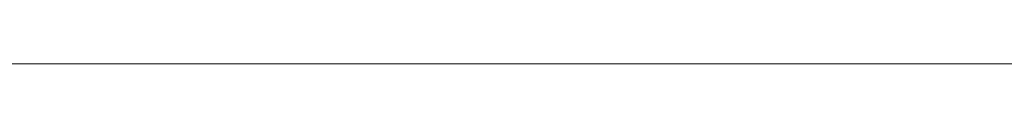
# Model space of a CAD drawing. Units: inches. Extents: x 459864 to 460310, y 324185 to 324787.
# Tile 87 of 112: x 460247.12218 to 460247.14006, y 324283.48322 to 324283.48324. Entities that reach past the tile are written whole.
import ezdxf

# ---------------------------------------------------------------- set-up
doc = ezdxf.new("R2010")
doc.units = ezdxf.units.IN
for name, color, linetype, lineweight in [('A-ANNO-DIMS', 2, 'Continuous', 18), ('L-HRDS', 9, 'Continuous', 18), ('L-SITE-PATT', 252, 'Continuous', 13)]:
    doc.layers.add(name, color=color, linetype=linetype, lineweight=lineweight)
doc.styles.get("Standard").update_dxf_attribs({"font": 'arial.ttf'})
doc.dimstyles.new('ISO-25', dxfattribs={"dimtxt": 6, "dimasz": 2.5, "dimexe": 1.25, "dimexo": 0.625, "dimtad": 1, "dimdec": 1, "dimlunit": 3, "dimtxsty": 'Standard', "dimcen": 2.5, "dimadec": 0, "dimazin": 0, "dimtfac": 1, "dimtdec": 1, "dimtmove": 0, "dimatfit": 3, "dimfxl": 1, "dimarcsym": 0})

# ---------------------------------------------------------------- blocks, each defined once
blk = doc.blocks.new('*D21')
at = {"layer": 'A-ANNO-DIMS', "color": 0, "lineweight": -2, "transparency": 16777216}
for p, q in [((460247.739927, 324715.483233), (460309.580369, 324715.483233)), ((460308.330369, 324712.983233), (460308.330369, 324285.983233)), ((460247.739927, 324283.483233), (460309.580369, 324283.483233))]:
    blk.add_line(p, q, dxfattribs=at)
at = {"layer": 'A-ANNO-DIMS', "color": 0, "transparency": 16777216}
for points in [[(460307.913702, 324712.983233), (460308.747035, 324712.983233), (460308.330369, 324715.483233)], [(460307.913702, 324285.983233), (460308.747035, 324285.983233), (460308.330369, 324283.483233)]]:
    blk.add_solid(points, dxfattribs=at)
at = {"layer": 'Defpoints', "color": 0, "transparency": 16777216}
for p in [(460247.114927, 324715.483233), (460247.114927, 324283.483233), (460308.330369, 324283.483233)]:
    blk.add_point(p, dxfattribs=at)
at = {"layer": 'A-ANNO-DIMS', "color": 0, "transparency": 16777216, "insert": (460304.639884, 324499.483233), "char_height": 6, "attachment_point": 5, "rotation": 90}
blk.add_mtext("36'", dxfattribs=at)

msp = doc.modelspace()

# ---------------------------------------------------------------- hatches: boundary and pattern name
at = {"layer": 'L-SITE-PATT'}
h = msp.add_hatch(dxfattribs=at)
h.set_pattern_fill('DOTS', color=256)
h.paths.add_polyline_path([(460269.803614, 324283.483233), (460247.114927, 324283.483233), (460121.929275, 324283.483233), (460121.929275, 324252.47302), (460117.429275, 324252.47302), (460110.123563, 324252.47302), (460110.123563, 324243.286537), (460080.829543, 324243.286537), (460080.829543, 324252.47302), (460061.114927, 324252.47302), (460061.114927, 324251.882422), (460077.9089, 324251.882422), (460077.9089, 324199.483233), (460080.829543, 324199.483233), (460080.829543, 324207.553216), (460110.123563, 324207.553216), (460110.123563, 324199.483233), (460110.813349, 324199.483233), (460262.114927, 324199.483233), (460269.803614, 324199.483233)], flags=17)
edge = h.paths.add_edge_path(flags=0)
edge.add_ellipse((460222.590295, 324263.813229), major_axis=(-8.485281, 8.485281), ratio=1, start_angle=405, end_angle=495, ccw=False)
edge.add_line((460214.820868, 324254.65989), (460214.831619, 324254.66592))
edge.add_ellipse((460222.590295, 324263.813229), major_axis=(-8.485281, 8.485281), ratio=1, start_angle=405, end_angle=495, ccw=False)
edge.add_line((460210.75891, 324261.780551), (460210.767583, 324261.786823))
edge.add_ellipse((460222.590295, 324263.813229), major_axis=(-8.485281, 8.485281), ratio=1, start_angle=405, end_angle=495, ccw=False)
edge.add_ellipse((460222.590295, 324263.813229), major_axis=(-8.485281, 8.485281), ratio=1, start_angle=392.754016, end_angle=405, ccw=False)
edge.add_ellipse((460222.590295, 324263.813229), major_axis=(-8.485281, 8.485281), ratio=1, start_angle=380.9347178, end_angle=392.754016, ccw=False)
edge.add_line((460211.337059, 324267.985029), (460211.340404, 324267.985029))
edge.add_ellipse((460222.590295, 324263.813229), major_axis=(-8.485281, 8.485281), ratio=1, start_angle=380.9347178, end_angle=392.754016, ccw=False)
edge.add_ellipse((460222.590295, 324263.813229), major_axis=(-8.485281, 8.485281), ratio=1, start_angle=347.9015209, end_angle=380.9347178, ccw=False)
edge.add_ellipse((460222.590295, 324263.813229), major_axis=(-8.485281, 8.485281), ratio=1, start_angle=327.0619241, end_angle=347.9015209, ccw=False)
edge.add_ellipse((460222.590295, 324263.813229), major_axis=(-8.485281, 8.485281), ratio=1, start_angle=278.3246418, end_angle=327.0619241, ccw=False)
edge.add_line((460225.158278, 324275.535991), (460225.157699, 324275.534637))
edge.add_ellipse((460222.590295, 324263.813229), major_axis=(-8.485281, 8.485281), ratio=1, start_angle=278.3246418, end_angle=327.0619241, ccw=False)
edge.add_ellipse((460222.590295, 324263.813229), major_axis=(-8.485281, 8.485281), ratio=1, start_angle=260.6435685, end_angle=278.3246418, ccw=False)
edge.add_ellipse((460222.590295, 324263.813229), major_axis=(-8.485281, 8.485281), ratio=1, start_angle=225, end_angle=260.6435685, ccw=False)
edge.add_line((460234.508791, 324265.242796), (460234.501456, 324265.239441))
edge.add_ellipse((460222.590295, 324263.813229), major_axis=(-8.485281, 8.485281), ratio=1, start_angle=225, end_angle=260.6435685, ccw=False)
edge.add_ellipse((460222.590295, 324263.813229), major_axis=(-8.485281, 8.485281), ratio=1, start_angle=495, end_angle=585, ccw=False)
edge.add_line((460234.436668, 324261.861215), (460234.423783, 324261.857822))
edge.add_ellipse((460222.590295, 324263.813229), major_axis=(-8.485281, 8.485281), ratio=1, start_angle=495, end_angle=585, ccw=False)
edge.add_line((460227.95013, 324253.067192), (460227.946414, 324253.083139))
edge.add_ellipse((460222.590295, 324263.813229), major_axis=(-8.485281, 8.485281), ratio=1, start_angle=495, end_angle=585, ccw=False)
edge.add_line((460226.222975, 324252.369267), (460226.21103, 324252.379551))
edge.add_ellipse((460222.590295, 324263.813229), major_axis=(-8.485281, 8.485281), ratio=1, start_angle=495, end_angle=585, ccw=False)
h.paths.add_polyline_path([(460219.651452, 324254.346654), (460218.461311, 324253.544985), (460218.275437, 324254.78932), (460219.642395, 324256.541765), (460219.62463, 324260.847564), (460216.110089, 324257.333022), (460214.349967, 324256.978066), (460215.416366, 324259.355678), (460212.523935, 324258.495823), (460213.137313, 324259.929797), (460218.507211, 324263.813229), (460222.590295, 324263.813229), (460222.590295, 324267.806698), (460218.175536, 324272.21231), (460219.025968, 324274.63898), (460222.590295, 324272.811129), (460222.590295, 324275.42332), (460223.057099, 324274.824931), (460222.67523, 324273.492211), (460225.911677, 324267.134611), (460219.62463, 324260.847564)], flags=0)
edge = h.paths.add_edge_path(flags=0)
edge.add_ellipse((460194.575758, 324264.046494), major_axis=(-8.485281, 8.485281), ratio=1, start_angle=495, end_angle=585, ccw=False)
edge.add_line((460199.935593, 324253.300458), (460199.931877, 324253.316405))
edge.add_ellipse((460194.575758, 324264.046494), major_axis=(-8.485281, 8.485281), ratio=1, start_angle=495, end_angle=585, ccw=False)
edge.add_line((460198.208438, 324252.602533), (460198.196493, 324252.612817))
edge.add_ellipse((460194.575758, 324264.046494), major_axis=(-8.485281, 8.485281), ratio=1, start_angle=495, end_angle=585, ccw=False)
edge.add_ellipse((460194.575758, 324264.046494), major_axis=(-8.485281, 8.485281), ratio=1, start_angle=405, end_angle=495, ccw=False)
edge.add_line((460186.806331, 324254.893156), (460186.817082, 324254.899186))
edge.add_ellipse((460194.575758, 324264.046494), major_axis=(-8.485281, 8.485281), ratio=1, start_angle=405, end_angle=495, ccw=False)
edge.add_line((460182.744373, 324262.013817), (460182.753046, 324262.020089))
edge.add_ellipse((460194.575758, 324264.046494), major_axis=(-8.485281, 8.485281), ratio=1, start_angle=405, end_angle=495, ccw=False)
edge.add_ellipse((460194.575758, 324264.046494), major_axis=(-8.485281, 8.485281), ratio=1, start_angle=392.754016, end_angle=405, ccw=False)
edge.add_ellipse((460194.575758, 324264.046494), major_axis=(-8.485281, 8.485281), ratio=1, start_angle=380.9347178, end_angle=392.754016, ccw=False)
edge.add_line((460183.322522, 324268.218294), (460183.325867, 324268.218294))
edge.add_ellipse((460194.575758, 324264.046494), major_axis=(-8.485281, 8.485281), ratio=1, start_angle=380.9347178, end_angle=392.754016, ccw=False)
edge.add_ellipse((460194.575758, 324264.046494), major_axis=(-8.485281, 8.485281), ratio=1, start_angle=347.9015209, end_angle=380.9347178, ccw=False)
edge.add_ellipse((460194.575758, 324264.046494), major_axis=(-8.485281, 8.485281), ratio=1, start_angle=327.0619241, end_angle=347.9015209, ccw=False)
edge.add_ellipse((460194.575758, 324264.046494), major_axis=(-8.485281, 8.485281), ratio=1, start_angle=278.3246418, end_angle=327.0619241, ccw=False)
edge.add_line((460197.143741, 324275.769257), (460197.143162, 324275.767903))
edge.add_ellipse((460194.575758, 324264.046494), major_axis=(-8.485281, 8.485281), ratio=1, start_angle=278.3246418, end_angle=327.0619241, ccw=False)
edge.add_ellipse((460194.575758, 324264.046494), major_axis=(-8.485281, 8.485281), ratio=1, start_angle=260.6435685, end_angle=278.3246418, ccw=False)
edge.add_ellipse((460194.575758, 324264.046494), major_axis=(-8.485281, 8.485281), ratio=1, start_angle=225, end_angle=260.6435685, ccw=False)
edge.add_line((460206.494254, 324265.476062), (460206.486919, 324265.472707))
edge.add_ellipse((460194.575758, 324264.046494), major_axis=(-8.485281, 8.485281), ratio=1, start_angle=225, end_angle=260.6435685, ccw=False)
edge.add_ellipse((460194.575758, 324264.046494), major_axis=(-8.485281, 8.485281), ratio=1, start_angle=495, end_angle=585, ccw=False)
edge.add_line((460206.422132, 324262.094481), (460206.409246, 324262.091088))
h.paths.add_polyline_path([(460191.610093, 324261.08083), (460191.636915, 324254.57992), (460190.446774, 324253.778251), (460190.2609, 324255.022585), (460191.627858, 324256.775031), (460191.610093, 324261.08083), (460188.095552, 324257.566288), (460186.33543, 324257.211332), (460187.40183, 324259.588944), (460184.509398, 324258.729088), (460185.122776, 324260.163063), (460190.492675, 324264.046494), (460194.575758, 324264.046494), (460194.575758, 324268.039963), (460190.160999, 324272.445576), (460191.011431, 324274.872246), (460194.575758, 324273.044395), (460194.575758, 324275.656585), (460195.042562, 324275.058197), (460194.660693, 324273.725477), (460197.897141, 324267.367877)], flags=0)
edge = h.paths.add_edge_path(flags=0)
edge.add_ellipse((460252.911961, 324263.577616), major_axis=(-8.485281, 8.485281), ratio=1, start_angle=405, end_angle=495, ccw=False)
edge.add_line((460241.080576, 324261.544938), (460241.089249, 324261.55121))
edge.add_ellipse((460252.911961, 324263.577616), major_axis=(-8.485281, 8.485281), ratio=1, start_angle=405, end_angle=495, ccw=False)
edge.add_ellipse((460252.911961, 324263.577616), major_axis=(-8.485281, 8.485281), ratio=1, start_angle=392.754016, end_angle=405, ccw=False)
edge.add_ellipse((460252.911961, 324263.577616), major_axis=(-8.485281, 8.485281), ratio=1, start_angle=380.9347178, end_angle=392.754016, ccw=False)
edge.add_line((460241.658725, 324267.749416), (460241.66207, 324267.749416))
edge.add_ellipse((460252.911961, 324263.577616), major_axis=(-8.485281, 8.485281), ratio=1, start_angle=380.9347178, end_angle=392.754016, ccw=False)
edge.add_ellipse((460252.911961, 324263.577616), major_axis=(-8.485281, 8.485281), ratio=1, start_angle=347.9015209, end_angle=380.9347178, ccw=False)
edge.add_ellipse((460252.911961, 324263.577616), major_axis=(-8.485281, 8.485281), ratio=1, start_angle=327.0619241, end_angle=347.9015209, ccw=False)
edge.add_ellipse((460252.911961, 324263.577616), major_axis=(-8.485281, 8.485281), ratio=1, start_angle=278.3246418, end_angle=327.0619241, ccw=False)
edge.add_line((460255.479944, 324275.300378), (460255.479365, 324275.299024))
edge.add_ellipse((460252.911961, 324263.577616), major_axis=(-8.485281, 8.485281), ratio=1, start_angle=278.3246418, end_angle=327.0619241, ccw=False)
edge.add_ellipse((460252.911961, 324263.577616), major_axis=(-8.485281, 8.485281), ratio=1, start_angle=260.6435685, end_angle=278.3246418, ccw=False)
edge.add_ellipse((460252.911961, 324263.577616), major_axis=(-8.485281, 8.485281), ratio=1, start_angle=225, end_angle=260.6435685, ccw=False)
edge.add_line((460264.830457, 324265.007183), (460264.823122, 324265.003828))
edge.add_ellipse((460252.911961, 324263.577616), major_axis=(-8.485281, 8.485281), ratio=1, start_angle=225, end_angle=260.6435685, ccw=False)
edge.add_ellipse((460252.911961, 324263.577616), major_axis=(-8.485281, 8.485281), ratio=1, start_angle=495, end_angle=585, ccw=False)
edge.add_line((460264.758335, 324261.625602), (460264.745449, 324261.622209))
edge.add_ellipse((460252.911961, 324263.577616), major_axis=(-8.485281, 8.485281), ratio=1, start_angle=495, end_angle=585, ccw=False)
edge.add_line((460258.271796, 324252.831579), (460258.268081, 324252.847526))
edge.add_ellipse((460252.911961, 324263.577616), major_axis=(-8.485281, 8.485281), ratio=1, start_angle=495, end_angle=585, ccw=False)
edge.add_line((460256.544641, 324252.133654), (460256.532696, 324252.143938))
edge.add_ellipse((460252.911961, 324263.577616), major_axis=(-8.485281, 8.485281), ratio=1, start_angle=495, end_angle=585, ccw=False)
edge.add_ellipse((460252.911961, 324263.577616), major_axis=(-8.485281, 8.485281), ratio=1, start_angle=405, end_angle=495, ccw=False)
edge.add_line((460245.142534, 324254.424277), (460245.153285, 324254.430307))
h.paths.add_polyline_path([(460244.671633, 324256.742453), (460245.738033, 324259.120065), (460242.845601, 324258.26021), (460243.458979, 324259.694184), (460248.828878, 324263.577616), (460252.911961, 324263.577616), (460252.911961, 324267.571085), (460248.497202, 324271.976697), (460249.347634, 324274.403367), (460252.911961, 324272.575516), (460252.911961, 324275.187707), (460253.378765, 324274.589318), (460252.996897, 324273.256598), (460256.233344, 324266.898998), (460249.946296, 324260.611951), (460249.973118, 324254.111041), (460248.782977, 324253.309372), (460248.597103, 324254.553707), (460249.964061, 324256.306152), (460249.946296, 324260.611951), (460246.431755, 324257.097409)], flags=0)
edge = h.paths.add_edge_path(flags=0)
edge.add_ellipse((460167.43869, 324262.832792), major_axis=(-8.485281, 8.485281), ratio=1, start_angle=495, end_angle=585, ccw=False)
edge.add_line((460172.798524, 324252.086755), (460172.794809, 324252.102702))
edge.add_ellipse((460167.43869, 324262.832792), major_axis=(-8.485281, 8.485281), ratio=1, start_angle=495, end_angle=585, ccw=False)
edge.add_line((460171.07137, 324251.38883), (460171.059425, 324251.399114))
edge.add_ellipse((460167.43869, 324262.832792), major_axis=(-8.485281, 8.485281), ratio=1, start_angle=495, end_angle=585, ccw=False)
edge.add_ellipse((460167.43869, 324262.832792), major_axis=(-8.485281, 8.485281), ratio=1, start_angle=405, end_angle=495, ccw=False)
edge.add_line((460159.669262, 324253.679453), (460159.680013, 324253.685483))
edge.add_ellipse((460167.43869, 324262.832792), major_axis=(-8.485281, 8.485281), ratio=1, start_angle=405, end_angle=495, ccw=False)
edge.add_line((460155.607304, 324260.800114), (460155.615977, 324260.806386))
edge.add_ellipse((460167.43869, 324262.832792), major_axis=(-8.485281, 8.485281), ratio=1, start_angle=405, end_angle=495, ccw=False)
edge.add_ellipse((460167.43869, 324262.832792), major_axis=(-8.485281, 8.485281), ratio=1, start_angle=392.754016, end_angle=405, ccw=False)
edge.add_ellipse((460167.43869, 324262.832792), major_axis=(-8.485281, 8.485281), ratio=1, start_angle=380.9347178, end_angle=392.754016, ccw=False)
edge.add_line((460156.185453, 324267.004592), (460156.188798, 324267.004592))
edge.add_ellipse((460167.43869, 324262.832792), major_axis=(-8.485281, 8.485281), ratio=1, start_angle=380.9347178, end_angle=392.754016, ccw=False)
edge.add_ellipse((460167.43869, 324262.832792), major_axis=(-8.485281, 8.485281), ratio=1, start_angle=347.9015209, end_angle=380.9347178, ccw=False)
edge.add_ellipse((460167.43869, 324262.832792), major_axis=(-8.485281, 8.485281), ratio=1, start_angle=327.0619241, end_angle=347.9015209, ccw=False)
edge.add_ellipse((460167.43869, 324262.832792), major_axis=(-8.485281, 8.485281), ratio=1, start_angle=278.3246418, end_angle=327.0619241, ccw=False)
edge.add_line((460170.006672, 324274.555554), (460170.006093, 324274.5542))
edge.add_ellipse((460167.43869, 324262.832792), major_axis=(-8.485281, 8.485281), ratio=1, start_angle=278.3246418, end_angle=327.0619241, ccw=False)
edge.add_ellipse((460167.43869, 324262.832792), major_axis=(-8.485281, 8.485281), ratio=1, start_angle=260.6435685, end_angle=278.3246418, ccw=False)
edge.add_ellipse((460167.43869, 324262.832792), major_axis=(-8.485281, 8.485281), ratio=1, start_angle=225, end_angle=260.6435685, ccw=False)
edge.add_line((460179.357186, 324264.262359), (460179.349851, 324264.259004))
edge.add_ellipse((460167.43869, 324262.832792), major_axis=(-8.485281, 8.485281), ratio=1, start_angle=225, end_angle=260.6435685, ccw=False)
edge.add_ellipse((460167.43869, 324262.832792), major_axis=(-8.485281, 8.485281), ratio=1, start_angle=495, end_angle=585, ccw=False)
edge.add_line((460179.285063, 324260.880778), (460179.272177, 324260.877385))
h.paths.add_polyline_path([(460164.473025, 324259.867127), (460164.499846, 324253.366217), (460163.309706, 324252.564548), (460163.123831, 324253.808883), (460164.49079, 324255.561328), (460164.473025, 324259.867127), (460160.958483, 324256.352585), (460159.198362, 324255.997629), (460160.264761, 324258.375241), (460157.372329, 324257.515386), (460157.985707, 324258.94936), (460163.355606, 324262.832792), (460167.43869, 324262.832792), (460167.43869, 324266.826261), (460163.02393, 324271.231873), (460163.874362, 324273.658543), (460167.43869, 324271.830692), (460167.43869, 324274.442883), (460167.905493, 324273.844494), (460167.523625, 324272.511774), (460170.760072, 324266.154174)], flags=0)
edge = h.paths.add_edge_path(flags=0)
edge.add_ellipse((460140.758089, 324262.369585), major_axis=(-8.485281, 8.485281), ratio=1, start_angle=495, end_angle=585, ccw=False)
edge.add_line((460146.117923, 324251.623548), (460146.114208, 324251.639495))
edge.add_ellipse((460140.758089, 324262.369585), major_axis=(-8.485281, 8.485281), ratio=1, start_angle=495, end_angle=585, ccw=False)
edge.add_line((460144.390769, 324250.925623), (460144.378824, 324250.935907))
edge.add_ellipse((460140.758089, 324262.369585), major_axis=(-8.485281, 8.485281), ratio=1, start_angle=495, end_angle=585, ccw=False)
edge.add_ellipse((460140.758089, 324262.369585), major_axis=(-8.485281, 8.485281), ratio=1, start_angle=405, end_angle=495, ccw=False)
edge.add_line((460132.988661, 324253.216246), (460132.999412, 324253.222276))
edge.add_ellipse((460140.758089, 324262.369585), major_axis=(-8.485281, 8.485281), ratio=1, start_angle=405, end_angle=495, ccw=False)
edge.add_line((460128.926703, 324260.336907), (460128.935376, 324260.343179))
edge.add_ellipse((460140.758089, 324262.369585), major_axis=(-8.485281, 8.485281), ratio=1, start_angle=405, end_angle=495, ccw=False)
edge.add_ellipse((460140.758089, 324262.369585), major_axis=(-8.485281, 8.485281), ratio=1, start_angle=392.754016, end_angle=405, ccw=False)
edge.add_ellipse((460140.758089, 324262.369585), major_axis=(-8.485281, 8.485281), ratio=1, start_angle=380.9347178, end_angle=392.754016, ccw=False)
edge.add_line((460129.504852, 324266.541385), (460129.508197, 324266.541385))
edge.add_ellipse((460140.758089, 324262.369585), major_axis=(-8.485281, 8.485281), ratio=1, start_angle=380.9347178, end_angle=392.754016, ccw=False)
edge.add_ellipse((460140.758089, 324262.369585), major_axis=(-8.485281, 8.485281), ratio=1, start_angle=347.9015209, end_angle=380.9347178, ccw=False)
edge.add_ellipse((460140.758089, 324262.369585), major_axis=(-8.485281, 8.485281), ratio=1, start_angle=327.0619241, end_angle=347.9015209, ccw=False)
edge.add_ellipse((460140.758089, 324262.369585), major_axis=(-8.485281, 8.485281), ratio=1, start_angle=278.3246418, end_angle=327.0619241, ccw=False)
edge.add_line((460143.326071, 324274.092347), (460143.325492, 324274.090993))
edge.add_ellipse((460140.758089, 324262.369585), major_axis=(-8.485281, 8.485281), ratio=1, start_angle=278.3246418, end_angle=327.0619241, ccw=False)
edge.add_ellipse((460140.758089, 324262.369585), major_axis=(-8.485281, 8.485281), ratio=1, start_angle=260.6435685, end_angle=278.3246418, ccw=False)
edge.add_ellipse((460140.758089, 324262.369585), major_axis=(-8.485281, 8.485281), ratio=1, start_angle=225, end_angle=260.6435685, ccw=False)
edge.add_line((460152.676585, 324263.799152), (460152.66925, 324263.795797))
edge.add_ellipse((460140.758089, 324262.369585), major_axis=(-8.485281, 8.485281), ratio=1, start_angle=225, end_angle=260.6435685, ccw=False)
edge.add_ellipse((460140.758089, 324262.369585), major_axis=(-8.485281, 8.485281), ratio=1, start_angle=495, end_angle=585, ccw=False)
edge.add_line((460152.604462, 324260.417571), (460152.591576, 324260.414178))
h.paths.add_polyline_path([(460137.792424, 324259.40392), (460137.819245, 324252.90301), (460136.629105, 324252.101341), (460136.44323, 324253.345676), (460137.810189, 324255.098121), (460137.792424, 324259.40392), (460134.277882, 324255.889378), (460132.517761, 324255.534422), (460133.58416, 324257.912034), (460130.691728, 324257.052179), (460131.305106, 324258.486153), (460136.675005, 324262.369585), (460140.758089, 324262.369585), (460140.758089, 324266.363054), (460136.343329, 324270.768666), (460137.193761, 324273.195336), (460140.758089, 324271.367485), (460140.758089, 324273.979676), (460141.224892, 324273.381287), (460140.843024, 324272.048567), (460144.079471, 324265.690967)], flags=0)
h.paths.add_polyline_path([(460110.123563, 324227.413868), (460080.829543, 324227.413868), (460080.829543, 324235.483851), (460110.123563, 324235.483851)], flags=16)
h.paths.add_polyline_path([(460110.123563, 324220.796634), (460110.123563, 324212.726651), (460080.829543, 324212.726651), (460080.829543, 324220.796634)], flags=16)
h.paths.add_polyline_path([(460269.803614, 324283.483233), (460247.114927, 324283.483233), (460121.929275, 324283.483233), (460121.929275, 324252.47302), (460117.429275, 324252.47302), (460110.123563, 324252.47302), (460110.123563, 324243.286537), (460080.829543, 324243.286537), (460080.829543, 324252.47302), (460061.114927, 324252.47302), (460061.114927, 324251.882422), (460077.9089, 324251.882422), (460077.9089, 324199.483233), (460080.829543, 324199.483233), (460080.829543, 324207.553216), (460110.123563, 324207.553216), (460110.123563, 324199.483233), (460262.114927, 324199.483233), (460269.803614, 324199.483233)], flags=17)
h.paths.add_polyline_path([(460219.651452, 324254.346654), (460218.461311, 324253.544985), (460218.275437, 324254.78932), (460219.642395, 324256.541765), (460219.62463, 324260.847564), (460216.110089, 324257.333022), (460214.349967, 324256.978066), (460215.416366, 324259.355678), (460212.523935, 324258.495823), (460213.137313, 324259.929797), (460218.507211, 324263.813229), (460222.590295, 324263.813229), (460220.180486, 324266.223037), (460215.460959, 324265.307646), (460211.834533, 324266.136551), (460216.246619, 324267.985029), (460218.418495, 324267.985029), (460222.590295, 324263.813229), (460222.590295, 324267.806698), (460218.175536, 324272.21231), (460219.025968, 324274.63898), (460222.590295, 324272.811129), (460222.590295, 324275.42332), (460223.057099, 324274.824931), (460222.67523, 324273.492211), (460225.911677, 324267.134611), (460222.590295, 324263.813229), (460231.382871, 324263.813229), (460228.484718, 324262.487825), (460224.425208, 324261.978316), (460228.679899, 324257.723625), (460228.965835, 324254.791014), (460227.141768, 324256.536632), (460227.542067, 324254.818575), (460227.333342, 324253.614466), (460222.590295, 324259.984626), (460222.590295, 324255.496666), (460221.377409, 324256.540849), (460220.575794, 324261.798728), (460219.62463, 324260.847564)], flags=0)
h.paths.add_polyline_path([(460199.127231, 324256.769898), (460199.52753, 324255.051841), (460199.318805, 324253.847732), (460194.575758, 324260.217892), (460194.575758, 324255.729932), (460193.362872, 324256.774115), (460192.561257, 324262.031993), (460191.610093, 324261.08083), (460191.636915, 324254.57992), (460190.446774, 324253.778251), (460190.2609, 324255.022585), (460191.627858, 324256.775031), (460191.610093, 324261.08083), (460188.095552, 324257.566288), (460186.33543, 324257.211332), (460187.40183, 324259.588944), (460184.509398, 324258.729088), (460185.122776, 324260.163063), (460190.492675, 324264.046494), (460194.575758, 324264.046494), (460192.16595, 324266.456303), (460187.446422, 324265.540912), (460183.819996, 324266.369816), (460188.232082, 324268.218294), (460190.403958, 324268.218294), (460194.575758, 324264.046494), (460194.575758, 324268.039963), (460190.160999, 324272.445576), (460191.011431, 324274.872246), (460194.575758, 324273.044395), (460194.575758, 324275.656585), (460195.042562, 324275.058197), (460194.660693, 324273.725477), (460197.897141, 324267.367877), (460194.575758, 324264.046494), (460203.368334, 324264.046494), (460200.470181, 324262.721091), (460196.410671, 324262.211582), (460200.665362, 324257.956891), (460200.951298, 324255.02428)], flags=0)
h.paths.add_polyline_path([(460244.671633, 324256.742453), (460245.738033, 324259.120065), (460242.845601, 324258.26021), (460243.458979, 324259.694184), (460248.828878, 324263.577616), (460252.911961, 324263.577616), (460250.502153, 324265.987424), (460245.782625, 324265.072033), (460242.156199, 324265.900938), (460246.568285, 324267.749416), (460248.740161, 324267.749416), (460252.911961, 324263.577616), (460252.911961, 324267.571085), (460248.497202, 324271.976697), (460249.347634, 324274.403367), (460252.911961, 324272.575516), (460252.911961, 324275.187707), (460253.378765, 324274.589318), (460252.996897, 324273.256598), (460256.233344, 324266.898998), (460252.911961, 324263.577616), (460261.704537, 324263.577616), (460258.806384, 324262.252212), (460254.746874, 324261.742703), (460259.001565, 324257.488012), (460259.287501, 324254.555401), (460257.463434, 324256.301019), (460257.863733, 324254.582962), (460257.655008, 324253.378853), (460252.911961, 324259.749013), (460252.911961, 324255.261053), (460251.699075, 324256.305236), (460250.89746, 324261.563115), (460249.946296, 324260.611951), (460249.973118, 324254.111041), (460248.782977, 324253.309372), (460248.597103, 324254.553707), (460249.964061, 324256.306152), (460249.946296, 324260.611951), (460246.431755, 324257.097409)], flags=0)
h.paths.add_polyline_path([(460173.528293, 324256.743188), (460173.81423, 324253.810577), (460171.990163, 324255.556195), (460172.390461, 324253.838138), (460172.181736, 324252.634029), (460167.43869, 324259.004189), (460167.43869, 324254.516229), (460166.225803, 324255.560412), (460165.424189, 324260.818291), (460164.473025, 324259.867127), (460164.499846, 324253.366217), (460163.309706, 324252.564548), (460163.123831, 324253.808883), (460164.49079, 324255.561328), (460164.473025, 324259.867127), (460160.958483, 324256.352585), (460159.198362, 324255.997629), (460160.264761, 324258.375241), (460157.372329, 324257.515386), (460157.985707, 324258.94936), (460163.355606, 324262.832792), (460167.43869, 324262.832792), (460165.028881, 324265.2426), (460160.309353, 324264.327209), (460156.682927, 324265.156114), (460161.095013, 324267.004592), (460163.26689, 324267.004592), (460167.43869, 324262.832792), (460167.43869, 324266.826261), (460163.02393, 324271.231873), (460163.874362, 324273.658543), (460167.43869, 324271.830692), (460167.43869, 324274.442883), (460167.905493, 324273.844494), (460167.523625, 324272.511774), (460170.760072, 324266.154174), (460167.43869, 324262.832792), (460176.231266, 324262.832792), (460173.333113, 324261.507388), (460169.273603, 324260.997879)], flags=0)
h.paths.add_polyline_path([(460146.847692, 324256.279981), (460147.133629, 324253.34737), (460145.309562, 324255.092988), (460145.70986, 324253.374931), (460145.501135, 324252.170822), (460140.758089, 324258.540983), (460140.758089, 324254.053022), (460139.545202, 324255.097205), (460138.743588, 324260.355084), (460137.792424, 324259.40392), (460137.819245, 324252.90301), (460136.629105, 324252.101341), (460136.44323, 324253.345676), (460137.810189, 324255.098121), (460137.792424, 324259.40392), (460134.277882, 324255.889378), (460132.517761, 324255.534422), (460133.58416, 324257.912034), (460130.691728, 324257.052179), (460131.305106, 324258.486153), (460136.675005, 324262.369585), (460140.758089, 324262.369585), (460138.34828, 324264.779393), (460133.628752, 324263.864002), (460130.002326, 324264.692907), (460134.414412, 324266.541385), (460136.586289, 324266.541385), (460140.758089, 324262.369585), (460140.758089, 324266.363054), (460136.343329, 324270.768666), (460137.193761, 324273.195336), (460140.758089, 324271.367485), (460140.758089, 324273.979676), (460141.224892, 324273.381287), (460140.843024, 324272.048567), (460144.079471, 324265.690967), (460140.758089, 324262.369585), (460149.550664, 324262.369585), (460146.652512, 324261.044182), (460142.593002, 324260.534672)], flags=0)
edge = h.paths.add_edge_path()
edge.add_line((460269.803614, 324272.549054), (460260.881484, 324272.549054))
edge.add_ellipse((460252.911961, 324263.577616), major_axis=(-8.485281, 8.485281), ratio=1, start_angle=260.6435685, end_angle=273.3846244, ccw=False)
edge.add_line((460262.282614, 324271.092108), (460262.260554, 324271.09106))
edge.add_ellipse((460252.911961, 324263.577616), major_axis=(-8.485281, 8.485281), ratio=1, start_angle=260.6435685, end_angle=273.3846244, ccw=False)
edge.add_ellipse((460252.911961, 324263.577616), major_axis=(-8.485281, 8.485281), ratio=1, start_angle=225, end_angle=260.6435685, ccw=False)
edge.add_line((460263.608568, 324269.063294), (460263.571652, 324269.058283))
edge.add_ellipse((460252.911961, 324263.577616), major_axis=(-8.485281, 8.485281), ratio=1, start_angle=225, end_angle=260.6435685, ccw=False)
edge.add_line((460264.615462, 324266.30554), (460264.585358, 324266.305196))
edge.add_ellipse((460252.911961, 324263.577616), major_axis=(-8.485281, 8.485281), ratio=1, start_angle=225, end_angle=260.6435685, ccw=False)
edge.add_line((460264.830457, 324265.007183), (460264.823122, 324265.003828))
edge.add_ellipse((460252.911961, 324263.577616), major_axis=(-8.485281, 8.485281), ratio=1, start_angle=225, end_angle=260.6435685, ccw=False)
edge.add_ellipse((460252.911961, 324263.577616), major_axis=(-8.485281, 8.485281), ratio=1, start_angle=495, end_angle=585, ccw=False)
edge.add_line((460264.758335, 324261.625602), (460264.745449, 324261.622209))
edge.add_ellipse((460252.911961, 324263.577616), major_axis=(-8.485281, 8.485281), ratio=1, start_angle=495, end_angle=585, ccw=False)
edge.add_line((460263.442202, 324257.739018), (460263.389259, 324257.779239))
edge.add_ellipse((460252.911961, 324263.577616), major_axis=(-8.485281, 8.485281), ratio=1, start_angle=495, end_angle=585, ccw=False)
edge.add_line((460258.128071, 324252.743505), (460258.101878, 324252.778683))
edge.add_ellipse((460252.911961, 324263.577616), major_axis=(-8.485281, 8.485281), ratio=1, start_angle=495, end_angle=585, ccw=False)
edge.add_line((460256.544641, 324252.133654), (460256.532696, 324252.143938))
edge.add_ellipse((460252.911961, 324263.577616), major_axis=(-8.485281, 8.485281), ratio=1, start_angle=495, end_angle=585, ccw=False)
edge.add_ellipse((460252.911961, 324263.577616), major_axis=(-8.485281, 8.485281), ratio=1, start_angle=405, end_angle=495, ccw=False)
edge.add_line((460250.593989, 324251.780412), (460250.604653, 324251.819817))
edge.add_ellipse((460252.911961, 324263.577616), major_axis=(-8.485281, 8.485281), ratio=1, start_angle=405, end_angle=495, ccw=False)
edge.add_line((460245.142534, 324254.424277), (460245.153285, 324254.430307))
edge.add_ellipse((460252.911961, 324263.577616), major_axis=(-8.485281, 8.485281), ratio=1, start_angle=405, end_angle=495, ccw=False)
edge.add_line((460243.524588, 324256.059004), (460243.560343, 324256.091361))
edge.add_ellipse((460252.911961, 324263.577616), major_axis=(-8.485281, 8.485281), ratio=1, start_angle=405, end_angle=495, ccw=False)
edge.add_line((460241.440103, 324259.892726), (460241.522441, 324259.895877))
edge.add_ellipse((460252.911961, 324263.577616), major_axis=(-8.485281, 8.485281), ratio=1, start_angle=405, end_angle=495, ccw=False)
edge.add_line((460241.080576, 324261.544938), (460241.089249, 324261.55121))
edge.add_ellipse((460252.911961, 324263.577616), major_axis=(-8.485281, 8.485281), ratio=1, start_angle=405, end_angle=495, ccw=False)
edge.add_ellipse((460252.911961, 324263.577616), major_axis=(-8.485281, 8.485281), ratio=1, start_angle=392.754016, end_angle=405, ccw=False)
edge.add_line((460241.050299, 324265.437612), (460241.062566, 324265.442751))
edge.add_ellipse((460252.911961, 324263.577616), major_axis=(-8.485281, 8.485281), ratio=1, start_angle=392.754016, end_angle=405, ccw=False)
edge.add_ellipse((460252.911961, 324263.577616), major_axis=(-8.485281, 8.485281), ratio=1, start_angle=380.9347178, end_angle=392.754016, ccw=False)
edge.add_line((460241.451888, 324267.176391), (460241.469044, 324267.170988))
edge.add_ellipse((460252.911961, 324263.577616), major_axis=(-8.485281, 8.485281), ratio=1, start_angle=380.9347178, end_angle=392.754016, ccw=False)
edge.add_line((460241.658725, 324267.749416), (460241.66207, 324267.749416))
edge.add_ellipse((460252.911961, 324263.577616), major_axis=(-8.485281, 8.485281), ratio=1, start_angle=380.9347178, end_angle=392.754016, ccw=False)
edge.add_ellipse((460252.911961, 324263.577616), major_axis=(-8.485281, 8.485281), ratio=1, start_angle=356.6153756, end_angle=380.9347178, ccw=False)
edge.add_line((460244.880293, 324272.487651), (460244.712651, 324272.549054))
edge.add_line((460244.712651, 324272.549054), (460230.817406, 324272.549054))
edge.add_ellipse((460222.590295, 324263.813229), major_axis=(-8.485281, 8.485281), ratio=1, start_angle=260.6435685, end_angle=271.7177746, ccw=False)
edge.add_ellipse((460222.590295, 324263.813229), major_axis=(-8.485281, 8.485281), ratio=1, start_angle=225, end_angle=260.6435685, ccw=False)
edge.add_line((460233.286902, 324269.298907), (460233.249986, 324269.293896))
edge.add_ellipse((460222.590295, 324263.813229), major_axis=(-8.485281, 8.485281), ratio=1, start_angle=225, end_angle=260.6435685, ccw=False)
edge.add_line((460234.293796, 324266.541153), (460234.263692, 324266.540809))
edge.add_ellipse((460222.590295, 324263.813229), major_axis=(-8.485281, 8.485281), ratio=1, start_angle=225, end_angle=260.6435685, ccw=False)
edge.add_line((460234.508791, 324265.242796), (460234.501456, 324265.239441))
edge.add_ellipse((460222.590295, 324263.813229), major_axis=(-8.485281, 8.485281), ratio=1, start_angle=225, end_angle=260.6435685, ccw=False)
edge.add_ellipse((460222.590295, 324263.813229), major_axis=(-8.485281, 8.485281), ratio=1, start_angle=495, end_angle=585, ccw=False)
edge.add_line((460234.436668, 324261.861215), (460234.423783, 324261.857822))
edge.add_ellipse((460222.590295, 324263.813229), major_axis=(-8.485281, 8.485281), ratio=1, start_angle=495, end_angle=585, ccw=False)
edge.add_line((460233.120535, 324257.974631), (460233.067593, 324258.014852))
edge.add_ellipse((460222.590295, 324263.813229), major_axis=(-8.485281, 8.485281), ratio=1, start_angle=495, end_angle=585, ccw=False)
edge.add_line((460227.806405, 324252.979118), (460227.780212, 324253.014296))
edge.add_ellipse((460222.590295, 324263.813229), major_axis=(-8.485281, 8.485281), ratio=1, start_angle=495, end_angle=585, ccw=False)
edge.add_line((460226.222975, 324252.369267), (460226.21103, 324252.379551))
edge.add_ellipse((460222.590295, 324263.813229), major_axis=(-8.485281, 8.485281), ratio=1, start_angle=495, end_angle=585, ccw=False)
edge.add_ellipse((460222.590295, 324263.813229), major_axis=(-8.485281, 8.485281), ratio=1, start_angle=405, end_angle=495, ccw=False)
edge.add_line((460220.272323, 324252.016025), (460220.282987, 324252.05543))
edge.add_ellipse((460222.590295, 324263.813229), major_axis=(-8.485281, 8.485281), ratio=1, start_angle=405, end_angle=495, ccw=False)
edge.add_line((460214.820868, 324254.65989), (460214.831619, 324254.66592))
edge.add_ellipse((460222.590295, 324263.813229), major_axis=(-8.485281, 8.485281), ratio=1, start_angle=405, end_angle=495, ccw=False)
edge.add_line((460213.202922, 324256.294617), (460213.238677, 324256.326974))
edge.add_ellipse((460222.590295, 324263.813229), major_axis=(-8.485281, 8.485281), ratio=1, start_angle=405, end_angle=495, ccw=False)
edge.add_line((460211.118437, 324260.128339), (460211.200774, 324260.13149))
edge.add_ellipse((460222.590295, 324263.813229), major_axis=(-8.485281, 8.485281), ratio=1, start_angle=405, end_angle=495, ccw=False)
edge.add_line((460210.75891, 324261.780551), (460210.767583, 324261.786823))
edge.add_ellipse((460222.590295, 324263.813229), major_axis=(-8.485281, 8.485281), ratio=1, start_angle=405, end_angle=495, ccw=False)
edge.add_ellipse((460222.590295, 324263.813229), major_axis=(-8.485281, 8.485281), ratio=1, start_angle=392.754016, end_angle=405, ccw=False)
edge.add_line((460210.728633, 324265.673225), (460210.7409, 324265.678364))
edge.add_ellipse((460222.590295, 324263.813229), major_axis=(-8.485281, 8.485281), ratio=1, start_angle=392.754016, end_angle=405, ccw=False)
edge.add_ellipse((460222.590295, 324263.813229), major_axis=(-8.485281, 8.485281), ratio=1, start_angle=380.9347178, end_angle=392.754016, ccw=False)
edge.add_line((460211.130222, 324267.412004), (460211.147378, 324267.406601))
edge.add_ellipse((460222.590295, 324263.813229), major_axis=(-8.485281, 8.485281), ratio=1, start_angle=380.9347178, end_angle=392.754016, ccw=False)
edge.add_line((460211.337059, 324267.985029), (460211.340404, 324267.985029))
edge.add_ellipse((460222.590295, 324263.813229), major_axis=(-8.485281, 8.485281), ratio=1, start_angle=380.9347178, end_angle=392.754016, ccw=False)
edge.add_ellipse((460222.590295, 324263.813229), major_axis=(-8.485281, 8.485281), ratio=1, start_angle=358.2822254, end_angle=380.9347178, ccw=False)
edge.add_line((460213.704522, 324271.901826), (460213.709044, 324271.868974))
edge.add_ellipse((460222.590295, 324263.813229), major_axis=(-8.485281, 8.485281), ratio=1, start_angle=358.2822254, end_angle=380.9347178, ccw=False)
edge.add_line((460214.363185, 324272.549054), (460203.078318, 324272.549054))
edge.add_line((460203.078318, 324272.549054), (460203.060342, 324272.531078))
edge.add_ellipse((460194.575758, 324264.046494), major_axis=(-8.485281, 8.485281), ratio=1, start_angle=260.6435685, end_angle=270.11679, ccw=False)
edge.add_line((460203.956591, 324271.56147), (460203.920907, 324271.559776))
edge.add_ellipse((460194.575758, 324264.046494), major_axis=(-8.485281, 8.485281), ratio=1, start_angle=260.6435685, end_angle=270.11679, ccw=False)
edge.add_ellipse((460194.575758, 324264.046494), major_axis=(-8.485281, 8.485281), ratio=1, start_angle=225, end_angle=260.6435685, ccw=False)
edge.add_line((460205.272365, 324269.532172), (460205.235449, 324269.527161))
edge.add_ellipse((460194.575758, 324264.046494), major_axis=(-8.485281, 8.485281), ratio=1, start_angle=225, end_angle=260.6435685, ccw=False)
edge.add_line((460206.279259, 324266.774419), (460206.249155, 324266.774075))
edge.add_ellipse((460194.575758, 324264.046494), major_axis=(-8.485281, 8.485281), ratio=1, start_angle=225, end_angle=260.6435685, ccw=False)
edge.add_line((460206.494254, 324265.476062), (460206.486919, 324265.472707))
edge.add_ellipse((460194.575758, 324264.046494), major_axis=(-8.485281, 8.485281), ratio=1, start_angle=225, end_angle=260.6435685, ccw=False)
edge.add_ellipse((460194.575758, 324264.046494), major_axis=(-8.485281, 8.485281), ratio=1, start_angle=495, end_angle=585, ccw=False)
edge.add_line((460206.422132, 324262.094481), (460206.409246, 324262.091088))
edge.add_ellipse((460194.575758, 324264.046494), major_axis=(-8.485281, 8.485281), ratio=1, start_angle=495, end_angle=585, ccw=False)
edge.add_line((460205.105999, 324258.207897), (460205.053056, 324258.248118))
edge.add_ellipse((460194.575758, 324264.046494), major_axis=(-8.485281, 8.485281), ratio=1, start_angle=495, end_angle=585, ccw=False)
edge.add_line((460199.791868, 324253.212383), (460199.765675, 324253.247562))
edge.add_ellipse((460194.575758, 324264.046494), major_axis=(-8.485281, 8.485281), ratio=1, start_angle=495, end_angle=585, ccw=False)
edge.add_line((460198.208438, 324252.602533), (460198.196493, 324252.612817))
edge.add_ellipse((460194.575758, 324264.046494), major_axis=(-8.485281, 8.485281), ratio=1, start_angle=495, end_angle=585, ccw=False)
edge.add_ellipse((460194.575758, 324264.046494), major_axis=(-8.485281, 8.485281), ratio=1, start_angle=405, end_angle=495, ccw=False)
edge.add_line((460192.257786, 324252.249291), (460192.26845, 324252.288696))
edge.add_ellipse((460194.575758, 324264.046494), major_axis=(-8.485281, 8.485281), ratio=1, start_angle=405, end_angle=495, ccw=False)
edge.add_line((460186.806331, 324254.893156), (460186.817082, 324254.899186))
edge.add_ellipse((460194.575758, 324264.046494), major_axis=(-8.485281, 8.485281), ratio=1, start_angle=405, end_angle=495, ccw=False)
edge.add_line((460185.188385, 324256.527883), (460185.22414, 324256.56024))
edge.add_ellipse((460194.575758, 324264.046494), major_axis=(-8.485281, 8.485281), ratio=1, start_angle=405, end_angle=495, ccw=False)
edge.add_line((460183.1039, 324260.361604), (460183.186238, 324260.364755))
edge.add_ellipse((460194.575758, 324264.046494), major_axis=(-8.485281, 8.485281), ratio=1, start_angle=405, end_angle=495, ccw=False)
edge.add_line((460182.744373, 324262.013817), (460182.753046, 324262.020089))
edge.add_ellipse((460194.575758, 324264.046494), major_axis=(-8.485281, 8.485281), ratio=1, start_angle=405, end_angle=495, ccw=False)
edge.add_ellipse((460194.575758, 324264.046494), major_axis=(-8.485281, 8.485281), ratio=1, start_angle=392.754016, end_angle=405, ccw=False)
edge.add_line((460182.714096, 324265.906491), (460182.726363, 324265.91163))
edge.add_ellipse((460194.575758, 324264.046494), major_axis=(-8.485281, 8.485281), ratio=1, start_angle=392.754016, end_angle=405, ccw=False)
edge.add_ellipse((460194.575758, 324264.046494), major_axis=(-8.485281, 8.485281), ratio=1, start_angle=380.9347178, end_angle=392.754016, ccw=False)
edge.add_line((460183.115685, 324267.645269), (460183.132841, 324267.639867))
edge.add_ellipse((460194.575758, 324264.046494), major_axis=(-8.485281, 8.485281), ratio=1, start_angle=380.9347178, end_angle=392.754016, ccw=False)
edge.add_line((460183.322522, 324268.218294), (460183.325867, 324268.218294))
edge.add_ellipse((460194.575758, 324264.046494), major_axis=(-8.485281, 8.485281), ratio=1, start_angle=380.9347178, end_angle=392.754016, ccw=False)
edge.add_ellipse((460194.575758, 324264.046494), major_axis=(-8.485281, 8.485281), ratio=1, start_angle=359.88321, end_angle=380.9347178, ccw=False)
edge.add_line((460184.491364, 324270.610774), (460184.553145, 324270.610774))
edge.add_ellipse((460194.575758, 324264.046494), major_axis=(-8.485281, 8.485281), ratio=1, start_angle=359.88321, end_angle=380.9347178, ccw=False)
edge.add_line((460185.345843, 324271.760239), (460185.378628, 324271.728015))
edge.add_ellipse((460194.575758, 324264.046494), major_axis=(-8.485281, 8.485281), ratio=1, start_angle=359.88321, end_angle=380.9347178, ccw=False)
edge.add_line((460185.696717, 324272.086185), (460185.632999, 324272.549054))
edge.add_line((460185.632999, 324272.549054), (460174.683448, 324272.549054))
edge.add_line((460174.683448, 324272.549054), (460174.606053, 324272.457183))
edge.add_ellipse((460167.43869, 324262.832792), major_axis=(-8.485281, 8.485281), ratio=1, start_angle=260.6435685, end_angle=278.3246418, ccw=False)
edge.add_ellipse((460167.43869, 324262.832792), major_axis=(-8.485281, 8.485281), ratio=1, start_angle=225, end_angle=260.6435685, ccw=False)
edge.add_line((460178.135297, 324268.31847), (460178.098381, 324268.313459))
edge.add_ellipse((460167.43869, 324262.832792), major_axis=(-8.485281, 8.485281), ratio=1, start_angle=225, end_angle=260.6435685, ccw=False)
edge.add_line((460179.14219, 324265.560716), (460179.112086, 324265.560372))
edge.add_ellipse((460167.43869, 324262.832792), major_axis=(-8.485281, 8.485281), ratio=1, start_angle=225, end_angle=260.6435685, ccw=False)
edge.add_line((460179.357186, 324264.262359), (460179.349851, 324264.259004))
edge.add_ellipse((460167.43869, 324262.832792), major_axis=(-8.485281, 8.485281), ratio=1, start_angle=225, end_angle=260.6435685, ccw=False)
edge.add_ellipse((460167.43869, 324262.832792), major_axis=(-8.485281, 8.485281), ratio=1, start_angle=495, end_angle=585, ccw=False)
edge.add_line((460179.285063, 324260.880778), (460179.272177, 324260.877385))
edge.add_ellipse((460167.43869, 324262.832792), major_axis=(-8.485281, 8.485281), ratio=1, start_angle=495, end_angle=585, ccw=False)
edge.add_line((460177.96893, 324256.994194), (460177.915987, 324257.034415))
edge.add_ellipse((460167.43869, 324262.832792), major_axis=(-8.485281, 8.485281), ratio=1, start_angle=495, end_angle=585, ccw=False)
edge.add_line((460172.654799, 324251.998681), (460172.628607, 324252.033859))
edge.add_ellipse((460167.43869, 324262.832792), major_axis=(-8.485281, 8.485281), ratio=1, start_angle=495, end_angle=585, ccw=False)
edge.add_line((460171.07137, 324251.38883), (460171.059425, 324251.399114))
edge.add_ellipse((460167.43869, 324262.832792), major_axis=(-8.485281, 8.485281), ratio=1, start_angle=495, end_angle=585, ccw=False)
edge.add_ellipse((460167.43869, 324262.832792), major_axis=(-8.485281, 8.485281), ratio=1, start_angle=405, end_angle=495, ccw=False)
edge.add_line((460165.120717, 324251.035588), (460165.131381, 324251.074993))
edge.add_ellipse((460167.43869, 324262.832792), major_axis=(-8.485281, 8.485281), ratio=1, start_angle=405, end_angle=495, ccw=False)
edge.add_line((460159.669262, 324253.679453), (460159.680013, 324253.685483))
edge.add_ellipse((460167.43869, 324262.832792), major_axis=(-8.485281, 8.485281), ratio=1, start_angle=405, end_angle=495, ccw=False)
edge.add_line((460158.051317, 324255.31418), (460158.087072, 324255.346537))
edge.add_ellipse((460167.43869, 324262.832792), major_axis=(-8.485281, 8.485281), ratio=1, start_angle=405, end_angle=495, ccw=False)
edge.add_line((460155.966831, 324259.147902), (460156.049169, 324259.151053))
edge.add_ellipse((460167.43869, 324262.832792), major_axis=(-8.485281, 8.485281), ratio=1, start_angle=405, end_angle=495, ccw=False)
edge.add_line((460155.607304, 324260.800114), (460155.615977, 324260.806386))
edge.add_ellipse((460167.43869, 324262.832792), major_axis=(-8.485281, 8.485281), ratio=1, start_angle=405, end_angle=495, ccw=False)
edge.add_ellipse((460167.43869, 324262.832792), major_axis=(-8.485281, 8.485281), ratio=1, start_angle=392.754016, end_angle=405, ccw=False)
edge.add_line((460155.577027, 324264.692788), (460155.589294, 324264.697927))
edge.add_ellipse((460167.43869, 324262.832792), major_axis=(-8.485281, 8.485281), ratio=1, start_angle=392.754016, end_angle=405, ccw=False)
edge.add_ellipse((460167.43869, 324262.832792), major_axis=(-8.485281, 8.485281), ratio=1, start_angle=380.9347178, end_angle=392.754016, ccw=False)
edge.add_line((460155.978616, 324266.431567), (460155.995772, 324266.426164))
edge.add_ellipse((460167.43869, 324262.832792), major_axis=(-8.485281, 8.485281), ratio=1, start_angle=380.9347178, end_angle=392.754016, ccw=False)
edge.add_line((460156.185453, 324267.004592), (460156.188798, 324267.004592))
edge.add_ellipse((460167.43869, 324262.832792), major_axis=(-8.485281, 8.485281), ratio=1, start_angle=380.9347178, end_angle=392.754016, ccw=False)
edge.add_ellipse((460167.43869, 324262.832792), major_axis=(-8.485281, 8.485281), ratio=1, start_angle=350.9344858, end_angle=380.9347178, ccw=False)
edge.add_line((460157.363277, 324269.397072), (460157.414394, 324269.397072))
edge.add_ellipse((460167.43869, 324262.832792), major_axis=(-8.485281, 8.485281), ratio=1, start_angle=350.9344858, end_angle=380.9347178, ccw=False)
edge.add_line((460158.220534, 324270.534977), (460158.236479, 324270.519306))
edge.add_ellipse((460167.43869, 324262.832792), major_axis=(-8.485281, 8.485281), ratio=1, start_angle=350.9344858, end_angle=380.9347178, ccw=False)
edge.add_line((460159.379443, 324271.752928), (460159.419308, 324271.738326))
edge.add_ellipse((460167.43869, 324262.832792), major_axis=(-8.485281, 8.485281), ratio=1, start_angle=350.9344858, end_angle=380.9347178, ccw=False)
edge.add_line((460160.396372, 324272.549054), (460147.112489, 324272.549054))
edge.add_ellipse((460140.758089, 324262.369585), major_axis=(-8.485281, 8.485281), ratio=1, start_angle=278.3246418, end_angle=283.0260712, ccw=False)
edge.add_ellipse((460140.758089, 324262.369585), major_axis=(-8.485281, 8.485281), ratio=1, start_angle=260.6435685, end_angle=278.3246418, ccw=False)
edge.add_ellipse((460140.758089, 324262.369585), major_axis=(-8.485281, 8.485281), ratio=1, start_angle=225, end_angle=260.6435685, ccw=False)
edge.add_line((460151.454695, 324267.855263), (460151.41778, 324267.850252))
edge.add_ellipse((460140.758089, 324262.369585), major_axis=(-8.485281, 8.485281), ratio=1, start_angle=225, end_angle=260.6435685, ccw=False)
edge.add_line((460152.461589, 324265.097509), (460152.431485, 324265.097165))
edge.add_ellipse((460140.758089, 324262.369585), major_axis=(-8.485281, 8.485281), ratio=1, start_angle=225, end_angle=260.6435685, ccw=False)
edge.add_line((460152.676585, 324263.799152), (460152.66925, 324263.795797))
edge.add_ellipse((460140.758089, 324262.369585), major_axis=(-8.485281, 8.485281), ratio=1, start_angle=225, end_angle=260.6435685, ccw=False)
edge.add_ellipse((460140.758089, 324262.369585), major_axis=(-8.485281, 8.485281), ratio=1, start_angle=495, end_angle=585, ccw=False)
edge.add_line((460152.604462, 324260.417571), (460152.591576, 324260.414178))
edge.add_ellipse((460140.758089, 324262.369585), major_axis=(-8.485281, 8.485281), ratio=1, start_angle=495, end_angle=585, ccw=False)
edge.add_line((460151.288329, 324256.530987), (460151.235386, 324256.571208))
edge.add_ellipse((460140.758089, 324262.369585), major_axis=(-8.485281, 8.485281), ratio=1, start_angle=495, end_angle=585, ccw=False)
edge.add_line((460145.974198, 324251.535474), (460145.948006, 324251.570652))
edge.add_ellipse((460140.758089, 324262.369585), major_axis=(-8.485281, 8.485281), ratio=1, start_angle=495, end_angle=585, ccw=False)
edge.add_line((460144.390769, 324250.925623), (460144.378824, 324250.935907))
edge.add_ellipse((460140.758089, 324262.369585), major_axis=(-8.485281, 8.485281), ratio=1, start_angle=495, end_angle=585, ccw=False)
edge.add_ellipse((460140.758089, 324262.369585), major_axis=(-8.485281, 8.485281), ratio=1, start_angle=405, end_angle=495, ccw=False)
edge.add_line((460138.440116, 324250.572381), (460138.45078, 324250.611786))
edge.add_ellipse((460140.758089, 324262.369585), major_axis=(-8.485281, 8.485281), ratio=1, start_angle=405, end_angle=495, ccw=False)
edge.add_line((460132.988661, 324253.216246), (460132.999412, 324253.222276))
edge.add_ellipse((460140.758089, 324262.369585), major_axis=(-8.485281, 8.485281), ratio=1, start_angle=405, end_angle=495, ccw=False)
edge.add_line((460131.370716, 324254.850973), (460131.40647, 324254.88333))
edge.add_ellipse((460140.758089, 324262.369585), major_axis=(-8.485281, 8.485281), ratio=1, start_angle=405, end_angle=495, ccw=False)
edge.add_line((460129.28623, 324258.684695), (460129.368568, 324258.687846))
edge.add_ellipse((460140.758089, 324262.369585), major_axis=(-8.485281, 8.485281), ratio=1, start_angle=405, end_angle=495, ccw=False)
edge.add_line((460128.926703, 324260.336907), (460128.935376, 324260.343179))
edge.add_ellipse((460140.758089, 324262.369585), major_axis=(-8.485281, 8.485281), ratio=1, start_angle=405, end_angle=495, ccw=False)
edge.add_ellipse((460140.758089, 324262.369585), major_axis=(-8.485281, 8.485281), ratio=1, start_angle=392.754016, end_angle=405, ccw=False)
edge.add_line((460128.896426, 324264.229581), (460128.908693, 324264.23472))
edge.add_ellipse((460140.758089, 324262.369585), major_axis=(-8.485281, 8.485281), ratio=1, start_angle=392.754016, end_angle=405, ccw=False)
edge.add_ellipse((460140.758089, 324262.369585), major_axis=(-8.485281, 8.485281), ratio=1, start_angle=380.9347178, end_angle=392.754016, ccw=False)
edge.add_line((460129.298015, 324265.96836), (460129.315171, 324265.962958))
edge.add_ellipse((460140.758089, 324262.369585), major_axis=(-8.485281, 8.485281), ratio=1, start_angle=380.9347178, end_angle=392.754016, ccw=False)
edge.add_line((460129.504852, 324266.541385), (460129.508197, 324266.541385))
edge.add_ellipse((460140.758089, 324262.369585), major_axis=(-8.485281, 8.485281), ratio=1, start_angle=380.9347178, end_angle=392.754016, ccw=False)
edge.add_ellipse((460140.758089, 324262.369585), major_axis=(-8.485281, 8.485281), ratio=1, start_angle=347.9015209, end_angle=380.9347178, ccw=False)
edge.add_line((460130.696859, 324268.933865), (460130.726822, 324268.933865))
edge.add_ellipse((460140.758089, 324262.369585), major_axis=(-8.485281, 8.485281), ratio=1, start_angle=347.9015209, end_angle=380.9347178, ccw=False)
edge.add_line((460131.869251, 324270.480437), (460131.87859, 324270.412595))
edge.add_ellipse((460140.758089, 324262.369585), major_axis=(-8.485281, 8.485281), ratio=1, start_angle=347.9015209, end_angle=380.9347178, ccw=False)
edge.add_line((460132.734121, 324271.276799), (460132.705361, 324271.287334))
edge.add_ellipse((460140.758089, 324262.369585), major_axis=(-8.485281, 8.485281), ratio=1, start_angle=347.9015209, end_angle=380.9347178, ccw=False)
edge.add_line((460134.239728, 324272.44485), (460134.203527, 324272.549054))
edge.add_line((460134.203527, 324272.549054), (460121.929275, 324272.549054))
edge.add_line((460121.929275, 324272.549054), (460121.929275, 324252.47302))
edge.add_line((460121.929275, 324252.47302), (460117.429275, 324252.47302))
edge.add_line((460117.429275, 324252.47302), (460110.123563, 324252.47302))
edge.add_line((460110.123563, 324252.47302), (460110.123563, 324243.286537))
edge.add_line((460110.123563, 324243.286537), (460080.829543, 324243.286537))
edge.add_line((460080.829543, 324243.286537), (460080.829543, 324252.47302))
edge.add_line((460080.829543, 324252.47302), (460061.114927, 324252.47302))
edge.add_line((460061.114927, 324252.47302), (460061.114927, 324251.882422))
edge.add_line((460061.114927, 324251.882422), (460077.9089, 324251.882422))
edge.add_line((460077.9089, 324251.882422), (460077.9089, 324199.483233))
edge.add_line((460077.9089, 324199.483233), (460080.829543, 324199.483233))
edge.add_line((460080.829543, 324199.483233), (460080.829543, 324207.553216))
edge.add_line((460080.829543, 324207.553216), (460110.123563, 324207.553216))
edge.add_line((460110.123563, 324207.553216), (460110.123563, 324199.483233))
edge.add_line((460110.123563, 324199.483233), (460110.813349, 324199.483233))
edge.add_line((460110.813349, 324199.483233), (460262.114927, 324199.483233))
edge.add_line((460262.114927, 324199.483233), (460269.803614, 324199.483233))
edge.add_line((460269.803614, 324199.483233), (460269.803614, 324272.549054))

# ---------------------------------------------------------------- linework, layer by layer
at = {"layer": 'L-HRDS'}
msp.add_line((460247.114927, 324283.483233), (460271.114927, 324283.483233), dxfattribs=at)

# ---------------------------------------------------------------- dimensions: what is measured, and where the dimension line sits
at = {"layer": 'A-ANNO-DIMS'}
dim = msp.add_linear_dim(base=(460308.330369, 324283.483233), p1=(460247.114927, 324715.483233), p2=(460247.114927, 324283.483233), angle=90, dimstyle='ISO-25', override={"dimclrd": 0, "dimclre": 0, "dimclrt": 0}, dxfattribs=at)
dim.commit()
dim.dimension.update_dxf_attribs({"geometry": '*D21', "text_midpoint": (460304.639884, 324499.483233)})

doc.saveas('drawing.dxf')
